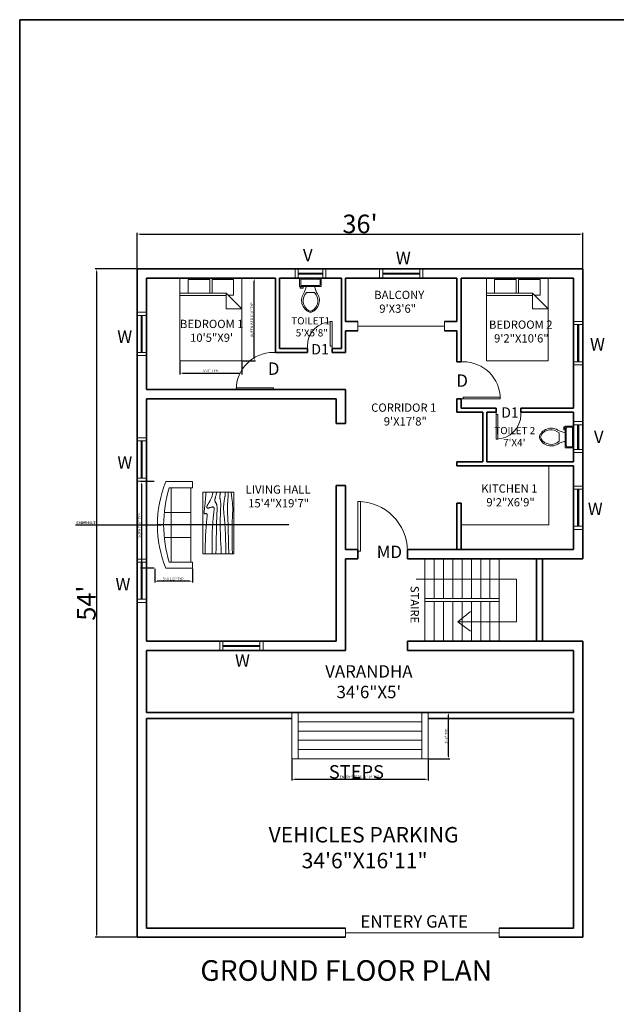
# Model space of a CAD drawing. Units: inches. Extents: x 2391 to 16591, y 7259 to 10239.
# Tile 19 of 27: x 2391 to 2970, y 9285 to 10239. Entities that reach past the tile are written whole.
import ezdxf

# ---------------------------------------------------------------- set-up
doc = ezdxf.new("R2010")
doc.units = ezdxf.units.IN
for name, color, linetype, lineweight in [('A-ANNO-DIMS', 4, 'Continuous', 18), ('A-ANNO-IDEN', 2, 'Continuous', 18), ('A-ANNO-SYMB', 3, 'Continuous', 18), ('A-ANNO-TITL', 3, 'Continuous', 30), ('A-ANNO-TTLB', 7, 'Continuous', 35), ('A-AREA-IDEN', 7, 'Continuous', 18), ('A-DOOR', 3, 'Continuous', 18), ('A-FLOR-CASE', 6, 'Continuous', 18), ('A-FLOR-FIXT', 9, 'Continuous', 18), ('A-FLOR-HRAL', 8, 'Continuous', 18), ('A-FLOR-STRS', 7, 'Continuous', 18), ('A-FURN', 8, 'Continuous', 18), ('A-GLAZ', 4, 'Continuous', 18), ('A-WALL', 7, 'Continuous', 35)]:
    doc.layers.add(name, color=color, linetype=linetype, lineweight=lineweight)
doc.styles.get("Standard").update_dxf_attribs({"font": 'arial.ttf'})
doc.dimstyles.new('ISO-25', dxfattribs={"dimtxt": 2.5, "dimasz": 2.5, "dimexe": 1.25, "dimexo": 0.625, "dimtad": 1, "dimdec": 0, "dimlunit": 3, "dimtxsty": 'Standard', "dimcen": 2.5, "dimadec": 0, "dimazin": 0, "dimtfac": 1, "dimtdec": 0, "dimtmove": 0, "dimatfit": 3, "dimfxl": 1, "dimarcsym": 0})

# ---------------------------------------------------------------- blocks, each defined once
blk = doc.blocks.new('*U11')
for p, q in [((-36, 0), (-36, 6)), ((0, 0), (0, 6))]:
    blk.add_line(p, q)
blk.add_lwpolyline([(0, 0), (0, -36), (-1.75, -36), (-1.75, 0)], close=True)
blk.add_arc((0, 0), 36, 180, 270)
blk = doc.blocks.new('*U8')
for p, q in [((-24, 0), (-24, -6)), ((0, 0), (0, -6))]:
    blk.add_line(p, q)
blk.add_lwpolyline([(0, 0), (0, 24), (-1.75, 24), (-1.75, 0)], close=True)
blk.add_arc((0, 0), 24, 90, 180)
blk = doc.blocks.new('*U12')
for p, q in [((0, 0), (0, -6)), ((-36, 0), (-36, -6))]:
    blk.add_line(p, q)
blk.add_lwpolyline([(0, 0), (0, 36), (-1.75, 36), (-1.75, 0)], close=True)
blk.add_arc((0, 0), 36, 90, 180)
blk = doc.blocks.new('*U9')
for p, q in [((0, 0), (0, 6)), ((24, 0), (24, 6))]:
    blk.add_line(p, q)
blk.add_lwpolyline([(0, 0), (0, -24), (1.75, -24), (1.75, 0)], close=True)
blk.add_arc((0, 0), 24, 270, 0)
blk = doc.blocks.new('*U18')
for p, q in [((0, 0), (0, -5)), ((32, 0), (32, -5))]:
    blk.add_line(p, q)
blk.add_lwpolyline([(0, 0), (0, 32), (1.75, 32), (1.75, 0)], close=True)
blk.add_arc((0, 0), 32, 0, 90)
blk = doc.blocks.new('Bed - Queen')
for p, q in [((0, -80.00003), (0, 0)), ((0, 0), (59.99999, 0)), ((59.99999, 0), (59.99999, -80.00003)), ((7.99999, -1.2), (28.79998, -1.2)), ((7.99999, -14.4), (7.99999, -1.2)), ((28.79998, -1.2), (28.79998, -14.4)), ((31.19999, -1.2), (51.99999, -1.2)), ((31.19999, -14.4), (31.19999, -1.2)), ((51.99999, -1.2), (51.99999, -16.4)), ((0, -14.4), (44.8, -14.4)), ((44.8, -16.8), (0, -16.8)), ((59.99999, -29.6), (44.8, -14.4)), ((44.8, -14.4), (44.8, -29.6)), ((51.99999, -16.4), (46.79936, -16.4)), ((44.8, -29.6), (59.99999, -29.6)), ((59.99999, -80.00003), (0, -80.00003))]:
    blk.add_line(p, q)
blk = doc.blocks.new('Toilet - top')
for p, q in [((-10, -8.5), (-8, -8.5)), ((-10, -9.5), (-10, -8.5)), ((-7, -9.5), (-10, -9.5)), ((-8, -8.5), (-8, -8)), ((-7, -8), (-7, -9.5)), ((-4, -8), (-6, -14)), ((4, -8), (6, -14)), ((9.5, -6), (9.5, -2)), ((4, -14), (-4, -14))]:
    blk.add_line(p, q)
blk.add_lwpolyline([(10.5, -8), (10.5, 0), (-10.5, 0), (-10.5, -8)], close=True)
for points in [[(-9.5, -2), (-9.5, -6)], [(8.5, -1), (-8.5, -1)], [(-8.5, -7), (8.5, -7)]]:
    blk.add_lwpolyline(points)
for centre, radius, start, end in [((-8.62, -1.88), 0.884, 81.8699, 188.1301), ((-8.62, -6.12), 0.884, 171.8699, 278.1301), ((8.62, -1.88), 0.884, 351.8699, 98.1301), ((8.62, -6.12), 0.884, 261.8699, 8.1301), ((3.52, -21.58), 12.17, 141.46911, 247.97143), ((4.2, -21.82), 11.33, 136.36773, 238.94682), ((-3.52, -21.58), 12.17, 292.02843, 38.53071), ((-4.2, -21.82), 11.33, 301.05301, 43.63209), ((0, -27.88), 4, 245.73182, 294.26817), ((0, -29), 4, 254.86053, 285.13947)]:
    blk.add_arc(centre, radius, start, end)
blk = doc.blocks.new('Sofa - Roundback 7 ft.')
for p, q in [((-12.00002, -32.4421), (-12.00003, -6.5971)), ((11.99997, -32.4421), (11.99998, -6.5971)), ((-36.000027, -34), (-36.000027, -11.4696)), ((-35.999844, -13.3819), (35.9998, -13.3819)), ((35.99998, -34), (35.99998, -11.4696)), ((-36.000027, -32.4421), (35.99998, -32.4421))]:
    blk.add_line(p, q)
for points in [[(-36.000027, -34), (-42.000027, -34), (-42.000027, -8)], [(41.99998, -8), (41.99998, -34), (35.99998, -34)]]:
    blk.add_lwpolyline(points)
for centre, radius, start, end in [((0, -114.25), 114.25, 68.43141, 111.5686), ((-0.00001, -127.1968), 121.1968, 72.72033, 107.2797)]:
    blk.add_arc(centre, radius, start, end)
blk = doc.blocks.new('Table - Rectangular Woodgrain 60 x 30 in.')
for p, q in [((0, 0), (0, -30)), ((60, 0), (0, 0)), ((60, -30), (60, 0)), ((0, -30), (60, -30))]:
    blk.add_line(p, q)
for points in [[(0, -2.4), (4.8155, -2.418), (9.0302, -2.4688), (12.709, -2.5477), (15.9167, -2.65), (18.7181, -2.7711), (21.1781, -2.9063), (23.3616, -3.0508), (25.3333, -3.2), (27.1477, -3.3495), (28.8172, -3.4958), (30.3437, -3.636), (31.7291, -3.7667), (32.9756, -3.8849), (34.0849, -3.9875), (35.059, -4.0714), (35.9, -4.1334), (36.6114, -4.1711), (37.2041, -4.1854), (37.6906, -4.1779), (38.0833, -4.15), (38.3948, -4.1034), (38.6375, -4.0396), (38.8239, -3.9602), (38.9666, -3.8667), (39.0764, -3.7608), (39.1573, -3.6448), (39.2116, -3.521), (39.2416, -3.3917), (39.2498, -3.2593), (39.2385, -3.1261), (39.21, -2.9944), (39.1666, -2.8667), (39.111, -2.7447), (39.0468, -2.6281), (38.978, -2.5163), (38.9083, -2.4083), (38.8418, -2.3035), (38.7823, -2.201), (38.7337, -2.1001), (38.7, -2), (38.6844, -1.9003), (38.6875, -1.8021), (38.7094, -1.707), (38.75, -1.6167), (38.8094, -1.5326), (38.8875, -1.4563), (38.9844, -1.3893), (39.1, -1.3333), (39.2351, -1.2896), (39.3937, -1.2583), (39.5804, -1.2396), (39.8, -1.2333), (40.057, -1.2396), (40.3562, -1.2583), (40.7023, -1.2896), (41.1, -1.3333), (41.5547, -1.3895), (42.0755, -1.4573), (42.6721, -1.5361), (43.3542, -1.625), (44.1316, -1.7233), (45.014, -1.8302), (46.0114, -1.9449), (47.1333, -2.0667), (48.3862, -2.1947), (49.7625, -2.3281), (51.2513, -2.4663), (52.8416, -2.6083), (54.5226, -2.7535), (56.2833, -2.9011), (58.1127, -3.0501), (60, -3.2)], [(0, -9.2), (6.5759, -9.0858), (11.9385, -9.0365), (16.2527, -9.0418), (19.6833, -9.0917), (22.3952, -9.1759), (24.5531, -9.2844), (26.322, -9.4069), (27.8666, -9.5333), (29.3241, -9.6553), (30.7203, -9.7719), (32.0532, -9.8837), (33.3208, -9.9917), (34.5213, -10.0965), (35.6526, -10.199), (36.7128, -10.2999), (37.7, -10.4), (38.6129, -10.4996), (39.4531, -10.5969), (40.223, -10.6895), (40.925, -10.775), (41.5613, -10.8512), (42.1344, -10.9156), (42.6465, -10.966), (43.1, -11), (43.4976, -11.0158), (43.8437, -11.0136), (44.143, -10.9942), (44.4, -10.9583), (44.6195, -10.9069), (44.8062, -10.8406), (44.9648, -10.7603), (45.1, -10.6667), (45.2155, -10.5598), (45.3114, -10.4365), (45.3871, -10.2929), (45.4416, -10.125), (45.4743, -9.929), (45.4844, -9.7011), (45.4709, -9.4371), (45.4333, -9.1333), (45.3716, -8.7883), (45.2896, -8.4104), (45.1919, -8.0107), (45.0833, -7.6), (44.9685, -7.1893), (44.8521, -6.7896), (44.7388, -6.4117), (44.6333, -6.0667), (44.54, -5.7628), (44.4614, -5.4979), (44.4001, -5.2675), (44.3583, -5.0667), (44.3384, -4.8909), (44.3427, -4.7354), (44.3736, -4.5956), (44.4333, -4.4667), (44.5236, -4.3453), (44.6427, -4.2333), (44.7884, -4.1339), (44.9583, -4.05), (45.1501, -3.9849), (45.3614, -3.9417), (45.59, -3.9234), (45.8333, -3.9333), (46.0915, -3.9749), (46.3734, -4.0531), (46.6906, -4.1736), (47.0542, -4.3417), (47.4756, -4.5629), (47.9661, -4.8427), (48.5372, -5.1866), (49.2, -5.6), (49.9676, -6.0844), (50.8594, -6.625), (51.8965, -7.2031), (53.1, -7.8), (54.491, -8.3969), (56.0906, -8.975), (57.9199, -9.5156), (60, -10)], [(0, -12.8), (5.1847, -12.9322), (9.6213, -13.0323), (13.3963, -13.1059), (16.5958, -13.1583), (19.3063, -13.1952), (21.614, -13.2219), (23.6054, -13.2439), (25.3666, -13.2667), (26.9728, -13.2947), (28.4531, -13.3281), (29.8256, -13.3663), (31.1083, -13.4083), (32.3191, -13.4535), (33.476, -13.501), (34.597, -13.5501), (35.7, -13.6), (36.7984, -13.6497), (37.8875, -13.6979), (38.9578, -13.743), (40, -13.7833), (41.0047, -13.8174), (41.9625, -13.8438), (42.864, -13.8607), (43.7, -13.8667), (44.4631, -13.8604), (45.1552, -13.8417), (45.7801, -13.8104), (46.3416, -13.7667), (46.8439, -13.7104), (47.2906, -13.6417), (47.6858, -13.5604), (48.0333, -13.4667), (48.3375, -13.3608), (48.6042, -13.2448), (48.8396, -13.121), (49.05, -12.9917), (49.2417, -12.8593), (49.4208, -12.7261), (49.5937, -12.5944), (49.7667, -12.4667), (49.9452, -12.3451), (50.1323, -12.2313), (50.3303, -12.1268), (50.5416, -12.0333), (50.7686, -11.9524), (51.0135, -11.8854), (51.2788, -11.8341), (51.5666, -11.8), (51.8785, -11.7843), (52.2116, -11.7865), (52.562, -11.8059), (52.926, -11.8417), (53.2998, -11.8931), (53.6795, -11.9594), (54.0614, -12.0397), (54.4416, -12.1333), (54.8223, -12.2401), (55.2293, -12.3625), (55.6942, -12.5037), (56.2489, -12.6667), (56.9251, -12.8547), (57.7545, -13.0708), (58.7689, -13.3182), (60, -13.6)], [(0, -18), (5.124, -17.7273), (9.6609, -17.5057), (13.6705, -17.3303), (17.2125, -17.1958), (20.3467, -17.0973), (23.1328, -17.0297), (25.6307, -16.9878), (27.9, -16.9667), (29.9928, -16.9617), (31.9302, -16.9703), (33.7254, -16.9907), (35.3917, -17.0208), (36.9423, -17.0588), (38.3906, -17.1026), (39.7499, -17.1503), (41.0333, -17.2), (42.2519, -17.2496), (43.4073, -17.2969), (44.4986, -17.3395), (45.525, -17.375), (46.4858, -17.4012), (47.3802, -17.4156), (48.2074, -17.416), (48.9667, -17.4), (49.6583, -17.3662), (50.2872, -17.3167), (50.8595, -17.2547), (51.3812, -17.1833), (51.8584, -17.1057), (52.2971, -17.025), (52.7034, -16.9443), (53.0833, -16.8667), (53.443, -16.7951), (53.789, -16.7313), (54.128, -16.6768), (54.4666, -16.6334), (54.8115, -16.6024), (55.1693, -16.5854), (55.5465, -16.5841), (55.95, -16.6), (56.3828, -16.6337), (56.8346, -16.6823), (57.2915, -16.7418), (57.7396, -16.8084), (58.165, -16.878), (58.5539, -16.9469), (58.8924, -17.0111), (59.1666, -17.0667), (59.3679, -17.1107), (59.5078, -17.1438), (59.6032, -17.1675), (59.6708, -17.1833), (59.7275, -17.193), (59.7901, -17.1979), (59.8753, -17.1998), (60, -17.2)], [(0, -22.4), (8.0098, -22.2501), (14.4094, -22.1011), (19.4168, -21.9535), (23.25, -21.8083), (26.1269, -21.6663), (28.2656, -21.5281), (29.884, -21.3947), (31.2, -21.2667), (32.3967, -21.1448), (33.5172, -21.0292), (34.5697, -20.9198), (35.5625, -20.8167), (36.5037, -20.7198), (37.4015, -20.6292), (38.2642, -20.5448), (39.1, -20.4667), (39.9164, -20.3951), (40.7187, -20.3313), (41.5117, -20.2768), (42.3, -20.2333), (43.0883, -20.2024), (43.8812, -20.1854), (44.6836, -20.1841), (45.5, -20.2), (46.3328, -20.234), (47.1747, -20.2844), (48.0163, -20.3488), (48.8479, -20.425), (49.66, -20.5106), (50.4429, -20.6031), (51.1872, -20.7004), (51.8833, -20.8), (52.5246, -20.8999), (53.1166, -20.9995), (53.6681, -21.0983), (54.1875, -21.1958), (54.6834, -21.2919), (55.1646, -21.3859), (55.6394, -21.4777), (56.1167, -21.5667), (56.6028, -21.6515), (57.0961, -21.7266), (57.5929, -21.7852), (58.0896, -21.8208), (58.5823, -21.8268), (59.0674, -21.7964), (59.5412, -21.723), (60, -21.6)], [(0, -25.2), (8.6355, -25.0504), (15.7026, -24.9031), (21.4049, -24.7606), (25.9458, -24.625), (29.529, -24.4988), (32.3578, -24.3844), (34.6359, -24.284), (36.5667, -24.2), (38.3213, -24.1341), (39.9417, -24.0854), (41.437, -24.0523), (42.8167, -24.0333), (44.0901, -24.0268), (45.2667, -24.0313), (46.3557, -24.0451), (47.3667, -24.0667), (48.309, -24.0947), (49.1928, -24.1287), (50.0284, -24.168), (50.826, -24.2125), (51.5959, -24.2617), (52.3483, -24.3151), (53.0935, -24.3725), (53.8417, -24.4334), (54.6009, -24.497), (55.3699, -24.561), (56.1454, -24.6226), (56.9239, -24.6792), (57.7021, -24.7279), (58.4764, -24.7662), (59.2435, -24.7911), (60, -24.8)], [(0, -28.8), (5.6867, -28.6681), (10.45, -28.5698), (14.407, -28.5012), (17.675, -28.4584), (20.3711, -28.4374), (22.6125, -28.4344), (24.5164, -28.4455), (26.2, -28.4667), (27.762, -28.4947), (29.2276, -28.5281), (30.6033, -28.5663), (31.8958, -28.6084), (33.1118, -28.6535), (34.2578, -28.7011), (35.3405, -28.7501), (36.3666, -28.8), (37.3443, -28.8497), (38.288, -28.8974), (39.2137, -28.9412), (40.1375, -28.9792), (41.0753, -29.0093), (42.0432, -29.0297), (43.0572, -29.0384), (44.1333, -29.0333), (45.2936, -29.0114), (46.5843, -28.9641), (48.0579, -28.8816), (49.7666, -28.7542), (51.7629, -28.5721), (54.0989, -28.3255), (56.8272, -28.0048), (60, -27.6)]]:
    blk.add_lwpolyline(points)
blk = doc.blocks.new('*D19')
at = {"layer": 'A-ANNO-DIMS', "color": 0, "lineweight": -2, "transparency": 16777216}
for p, q in [((2505.16, 9998.38), (2505.16, 10032.8)), ((2937.16, 9998.38), (2937.16, 10032.8)), ((2507.66, 10031.55), (2934.66, 10031.55))]:
    blk.add_line(p, q, dxfattribs=at)
at = {"layer": 'A-ANNO-DIMS', "color": 0, "transparency": 16777216}
for points in [[(2507.66, 10031.97), (2507.66, 10031.14), (2505.16, 10031.55)], [(2934.66, 10031.97), (2934.66, 10031.14), (2937.16, 10031.55)]]:
    blk.add_solid(points, dxfattribs=at)
at = {"layer": 'Defpoints', "color": 0, "transparency": 16777216}
for p in [(2937.16, 10031.55), (2505.16, 9997.76), (2937.16, 9997.76)]:
    blk.add_point(p, dxfattribs=at)
at = {"layer": 'A-ANNO-DIMS', "color": 0, "transparency": 16777216, "insert": (2721.16, 10041.38), "char_height": 2.5, "attachment_point": 5}
blk.add_mtext("{\\H7.2x;36'}", dxfattribs=at)
blk = doc.blocks.new('*D20')
at = {"layer": 'A-ANNO-DIMS', "color": 0, "lineweight": -2, "transparency": 16777216}
for p, q in [((2504.54, 9997.76), (2464.45, 9997.76)), ((2465.7, 9995.26), (2465.7, 9352.26)), ((2504.54, 9349.76), (2464.45, 9349.76))]:
    blk.add_line(p, q, dxfattribs=at)
at = {"layer": 'A-ANNO-DIMS', "color": 0, "transparency": 16777216}
for points in [[(2465.28, 9995.26), (2466.11, 9995.26), (2465.7, 9997.76)], [(2465.28, 9352.26), (2466.11, 9352.26), (2465.7, 9349.76)]]:
    blk.add_solid(points, dxfattribs=at)
at = {"layer": 'Defpoints', "color": 0, "transparency": 16777216}
for p in [(2505.16, 9997.76), (2465.7, 9349.76), (2505.16, 9349.76)]:
    blk.add_point(p, dxfattribs=at)
at = {"layer": 'A-ANNO-DIMS', "color": 0, "transparency": 16777216, "insert": (2455.92, 9673.76), "char_height": 2.5, "attachment_point": 5, "rotation": 90}
blk.add_mtext("{\\H7.2x;54'}", dxfattribs=at)
blk = doc.blocks.new('WINDOW-36-PLAN')
for p, q in [((9, 42), (0, 42)), ((9, 39), (0, 39)), ((4, 39), (4, 3)), ((4.5, 39), (4.5, 3)), ((5, 39), (5, 3)), ((9, 3), (0, 3)), ((9, 0), (0, 0))]:
    blk.add_line(p, q)
blk = doc.blocks.new('VENT-24-PLAN')
for p, q in [((9, 30), (0, 30)), ((9, 27), (0, 27)), ((4, 27), (4, 3)), ((4.5, 27), (4.5, 3)), ((5, 27), (5, 3)), ((9, 3), (0, 3)), ((9, 0), (0, 0))]:
    blk.add_line(p, q)
blk = doc.blocks.new('STAIR-RETURN-FLIGHT')
for p, q in [((0, 80), (0, 0)), ((9, 80), (9, 41.5)), ((18, 80), (18, 41.5)), ((27, 80), (27, 41.5)), ((36, 80), (36, 41.5)), ((45, 80), (45, 41.5)), ((54, 80), (54, 41.5)), ((63, 80), (63, 41.5)), ((72, 80), (72, 0)), ((72, 41.5), (0, 41.5)), ((72, 38.5), (0, 38.5)), ((9, 38.5), (9, 0)), ((18, 38.5), (18, 0)), ((27, 38.5), (27, 0)), ((36, 38.5), (36, 0)), ((45, 38.5), (45, 0)), ((54, 38.5), (54, 0)), ((63, 38.5), (63, 0))]:
    blk.add_line(p, q)
blk = doc.blocks.new('STAIR-DIRECTION-ARROW')
for p, q in [((0, 50.31), (97.37, 50.31)), ((97.37, 50.31), (97.37, 8.81)), ((40.34, 8.81), (52.74, 18.89)), ((97.37, 8.81), (40.34, 8.81)), ((40.34, 8.81), (52.74, 0))]:
    blk.add_line(p, q)
blk = doc.blocks.new('COUNTER-L-KITCHEN-TYPE2')
for p in [(85, 57), (0, 0)]:
    blk.add_line(p, (85, 0))
blk = doc.blocks.new('STAIR-ENTRY-STEPS')
for p, q in [((0, 45), (0, 0)), ((6, 45), (6, 0)), ((126, 45), (126, 0)), ((132, 45), (132, 0)), ((6, 36), (126, 36)), ((6, 27), (126, 27)), ((6, 18), (126, 18)), ((6, 9), (126, 9)), ((0, 0), (132, 0))]:
    blk.add_line(p, q)
blk = doc.blocks.new('*D45')
at = {"layer": 'A-ANNO-DIMS', "color": 0, "lineweight": -2, "transparency": 16777216}
for p, q in [((2607.29, 9988.76), (2619.91, 9988.76)), ((2618.66, 9911.26), (2618.66, 9986.26)), ((2607.29, 9908.76), (2619.91, 9908.76))]:
    blk.add_line(p, q, dxfattribs=at)
at = {"layer": 'A-ANNO-DIMS', "color": 0, "transparency": 16777216}
for points in [[(2618.24, 9986.26), (2619.08, 9986.26), (2618.66, 9988.76)], [(2618.24, 9911.26), (2619.08, 9911.26), (2618.66, 9908.76)]]:
    blk.add_solid(points, dxfattribs=at)
at = {"layer": 'Defpoints', "color": 0, "transparency": 16777216}
for p in [(2606.66, 9988.76), (2618.66, 9988.76), (2606.66, 9908.76)]:
    blk.add_point(p, dxfattribs=at)
at = {"layer": 'A-ANNO-DIMS', "color": 0, "transparency": 16777216, "insert": (2616.67, 9948.76), "char_height": 2.5, "attachment_point": 5, "rotation": 90}
blk.add_mtext('QUEEN BED 6\'-8" TYP.', dxfattribs=at)
blk = doc.blocks.new('*D46')
at = {"layer": 'A-ANNO-DIMS', "color": 0, "lineweight": -2, "transparency": 16777216}
for p, q in [((2546.66, 9908.13), (2546.66, 9895.51)), ((2606.66, 9908.13), (2606.66, 9895.51)), ((2549.16, 9896.76), (2604.16, 9896.76))]:
    blk.add_line(p, q, dxfattribs=at)
at = {"layer": 'A-ANNO-DIMS', "color": 0, "transparency": 16777216}
for points in [[(2549.16, 9897.17), (2549.16, 9896.34), (2546.66, 9896.76)], [(2604.16, 9897.17), (2604.16, 9896.34), (2606.66, 9896.76)]]:
    blk.add_solid(points, dxfattribs=at)
at = {"layer": 'Defpoints', "color": 0, "transparency": 16777216}
for p in [(2546.66, 9908.76), (2606.66, 9908.76), (2606.66, 9896.76)]:
    blk.add_point(p, dxfattribs=at)
at = {"layer": 'A-ANNO-DIMS', "color": 0, "transparency": 16777216, "insert": (2576.66, 9898.66), "char_height": 2.5, "attachment_point": 5}
blk.add_mtext('5\'-0" TYP.', dxfattribs=at)
blk = doc.blocks.new('*D49')
at = {"layer": 'A-ANNO-DIMS', "color": 0, "lineweight": -2, "transparency": 16777216}
for p, q in [((2521.54, 9791.53), (2508.32, 9791.53)), ((2509.57, 9710.03), (2509.57, 9789.03)), ((2521.54, 9707.53), (2508.32, 9707.53))]:
    blk.add_line(p, q, dxfattribs=at)
at = {"layer": 'A-ANNO-DIMS', "color": 0, "transparency": 16777216}
for points in [[(2509.15, 9789.03), (2509.98, 9789.03), (2509.57, 9791.53)], [(2509.15, 9710.03), (2509.98, 9710.03), (2509.57, 9707.53)]]:
    blk.add_solid(points, dxfattribs=at)
at = {"layer": 'Defpoints', "color": 0, "transparency": 16777216}
for p in [(2509.57, 9791.53), (2522.17, 9791.53), (2522.17, 9707.53)]:
    blk.add_point(p, dxfattribs=at)
at = {"layer": 'A-ANNO-DIMS', "color": 0, "transparency": 16777216, "insert": (2507.65, 9749.53), "char_height": 2.5, "attachment_point": 5, "rotation": 90}
blk.add_mtext('SOFA 7\'-0" TYP.', dxfattribs=at)
blk = doc.blocks.new('*D50')
at = {"layer": 'A-ANNO-DIMS', "color": 0, "lineweight": -2, "transparency": 16777216}
for p, q in [((2522.17, 9706.91), (2522.17, 9693.68)), ((2558.83, 9706.91), (2558.83, 9693.68)), ((2556.33, 9694.93), (2524.67, 9694.93))]:
    blk.add_line(p, q, dxfattribs=at)
at = {"layer": 'A-ANNO-DIMS', "color": 0, "transparency": 16777216}
for points in [[(2524.67, 9695.35), (2524.67, 9694.52), (2522.17, 9694.93)], [(2556.33, 9695.35), (2556.33, 9694.52), (2558.83, 9694.93)]]:
    blk.add_solid(points, dxfattribs=at)
at = {"layer": 'Defpoints', "color": 0, "transparency": 16777216}
for p in [(2522.17, 9707.53), (2558.83, 9707.53), (2522.17, 9694.93)]:
    blk.add_point(p, dxfattribs=at)
at = {"layer": 'A-ANNO-DIMS', "color": 0, "transparency": 16777216, "insert": (2540.5, 9696.85), "char_height": 2.5, "attachment_point": 5}
blk.add_mtext('3\'-0 1/2" TYP.', dxfattribs=at)
blk = doc.blocks.new('*D61')
at = {"layer": 'A-ANNO-DIMS', "color": 0, "lineweight": -2, "transparency": 16777216}
for p, q in [((2655.16, 9522.13), (2655.16, 9501.71)), ((2787.16, 9522.13), (2787.16, 9501.71)), ((2657.66, 9502.96), (2784.66, 9502.96))]:
    blk.add_line(p, q, dxfattribs=at)
at = {"layer": 'A-ANNO-DIMS', "color": 0, "transparency": 16777216}
for points in [[(2657.66, 9503.37), (2657.66, 9502.54), (2655.16, 9502.96)], [(2784.66, 9503.37), (2784.66, 9502.54), (2787.16, 9502.96)]]:
    blk.add_solid(points, dxfattribs=at)
at = {"layer": 'Defpoints', "color": 0, "transparency": 16777216}
for p in [(2655.16, 9522.76), (2787.16, 9522.76), (2787.16, 9502.96)]:
    blk.add_point(p, dxfattribs=at)
at = {"layer": 'A-ANNO-DIMS', "color": 0, "transparency": 16777216, "insert": (2721.16, 9504.88), "char_height": 2.5, "attachment_point": 5}
blk.add_mtext('ENTRY STEPS 11\'-0" TYP.', dxfattribs=at)
blk = doc.blocks.new('*D62')
at = {"layer": 'A-ANNO-DIMS', "color": 0, "lineweight": -2, "transparency": 16777216}
for p, q in [((2787.79, 9567.76), (2808.21, 9567.76)), ((2806.96, 9525.26), (2806.96, 9565.26)), ((2787.79, 9522.76), (2808.21, 9522.76))]:
    blk.add_line(p, q, dxfattribs=at)
at = {"layer": 'A-ANNO-DIMS', "color": 0, "transparency": 16777216}
for points in [[(2806.54, 9565.26), (2807.38, 9565.26), (2806.96, 9567.76)], [(2806.54, 9525.26), (2807.38, 9525.26), (2806.96, 9522.76)]]:
    blk.add_solid(points, dxfattribs=at)
at = {"layer": 'Defpoints', "color": 0, "transparency": 16777216}
for p in [(2787.16, 9567.76), (2806.96, 9567.76), (2787.16, 9522.76)]:
    blk.add_point(p, dxfattribs=at)
at = {"layer": 'A-ANNO-DIMS', "color": 0, "transparency": 16777216, "insert": (2805.06, 9545.26), "char_height": 2.5, "attachment_point": 5, "rotation": 90}
blk.add_mtext('3\'-9" TYP.', dxfattribs=at)
blk = doc.blocks.new('*D117')
at = {"layer": 'A-ANNO-DIMS', "color": 0, "lineweight": -2, "transparency": 16777216}
for p, q in [((2449.31, 9749.53), (2528.33, 9749.53)), ((2652.03, 9749.53), (2530.83, 9749.53))]:
    blk.add_line(p, q, dxfattribs=at)
at = {"layer": 'A-ANNO-DIMS', "color": 0, "transparency": 16777216}
blk.add_solid([(2528.33, 9749.95), (2528.33, 9749.11), (2530.83, 9749.53)], dxfattribs=at)
at = {"layer": 'Defpoints', "color": 0, "transparency": 16777216}
for p in [(2530.83, 9749.53), (2652.03, 9749.53)]:
    blk.add_point(p, dxfattribs=at)
at = {"layer": 'A-ANNO-DIMS', "color": 0, "transparency": 16777216, "insert": (2458.11, 9751.43), "char_height": 2.5, "attachment_point": 5, "rotation": 0.00135}
blk.add_mtext('6X R10\'-1"', dxfattribs=at)
blk = doc.blocks.new('*D118')
at = {"layer": 'A-ANNO-DIMS', "color": 0, "lineweight": -2, "transparency": 16777216}
for p, q in [((2445.53, 9749.53), (2522.33, 9749.53)), ((2639.08, 9749.53), (2524.83, 9749.53))]:
    blk.add_line(p, q, dxfattribs=at)
at = {"layer": 'A-ANNO-DIMS', "color": 0, "transparency": 16777216}
blk.add_solid([(2522.33, 9749.95), (2522.33, 9749.11), (2524.83, 9749.53)], dxfattribs=at)
at = {"layer": 'Defpoints', "color": 0, "transparency": 16777216}
for p in [(2524.83, 9749.53), (2639.08, 9749.53)]:
    blk.add_point(p, dxfattribs=at)
at = {"layer": 'A-ANNO-DIMS', "color": 0, "transparency": 16777216, "insert": (2456.28, 9751.45), "char_height": 2.5, "attachment_point": 5, "rotation": 0.00144}
blk.add_mtext('6X R9\'-6 1/2"', dxfattribs=at)

msp = doc.modelspace()

# ---------------------------------------------------------------- linework, layer by layer
at = {"layer": 'A-ANNO-TTLB'}
msp.add_lwpolyline([(2391.28, 10239.38), (4154.2, 10239.38), (4154.2, 7258.54), (2391.28, 7258.54)], close=True, dxfattribs=at)
at = {"layer": 'A-DOOR'}
for p, q in [((2707.16, 9358.76), (2707.16, 9349.76)), ((2856.16, 9358.76), (2856.16, 9349.76)), ((2707.16, 9354.26), (2856.16, 9354.26))]:
    msp.add_line(p, q, dxfattribs=at)
at = {"layer": 'A-FLOR-HRAL'}
for p, q in [((2719.16, 9937.76), (2719.16, 9946.76)), ((2803.16, 9937.76), (2803.16, 9946.76)), ((2719.16, 9942.26), (2803.16, 9942.26))]:
    msp.add_line(p, q, dxfattribs=at)
at = {"layer": 'A-WALL'}
for p, q in [((2505.16, 9997.76), (2937.16, 9997.76)), ((2505.16, 9349.76), (2505.16, 9997.76)), ((2937.16, 9997.76), (2937.16, 9716.76)), ((2514.16, 9988.76), (2639.16, 9988.76)), ((2514.16, 9880.76), (2514.16, 9988.76)), ((2639.16, 9916.76), (2639.16, 9988.76)), ((2643.16, 9920.76), (2643.16, 9988.76)), ((2643.16, 9988.76), (2703.16, 9988.76)), ((2703.16, 9920.76), (2703.16, 9988.76)), ((2707.16, 9988.76), (2815.16, 9988.76)), ((2707.16, 9946.76), (2707.16, 9988.76)), ((2815.16, 9946.76), (2815.16, 9988.76)), ((2819.16, 9988.76), (2928.16, 9988.76)), ((2819.16, 9907.76), (2819.16, 9988.76)), ((2928.16, 9988.76), (2928.16, 9862.76)), ((2707.16, 9946.76), (2719.16, 9946.76)), ((2803.16, 9946.76), (2815.16, 9946.76)), ((2707.16, 9916.76), (2707.16, 9937.76)), ((2707.16, 9937.76), (2719.16, 9937.76)), ((2803.16, 9937.76), (2815.16, 9937.76)), ((2815.16, 9907.76), (2815.16, 9937.76)), ((2643.16, 9920.76), (2670.16, 9920.76)), ((2670.16, 9916.76), (2670.16, 9920.76)), ((2694.16, 9916.76), (2694.16, 9920.76)), ((2694.16, 9920.76), (2703.16, 9920.76)), ((2639.16, 9916.76), (2670.16, 9916.76)), ((2694.16, 9916.76), (2707.16, 9916.76)), ((2815.16, 9907.76), (2819.16, 9907.76)), ((2514.16, 9880.76), (2707.16, 9880.76)), ((2707.16, 9847.76), (2707.16, 9880.76)), ((2514.16, 9871.76), (2698.16, 9871.76)), ((2514.16, 9636.76), (2514.16, 9871.76)), ((2698.16, 9847.76), (2698.16, 9871.76)), ((2815.16, 9858.76), (2815.16, 9871.76)), ((2815.16, 9871.76), (2819.16, 9871.76)), ((2819.16, 9862.76), (2819.16, 9871.76)), ((2819.16, 9862.76), (2853.16, 9862.76)), ((2853.16, 9862.76), (2853.16, 9858.76)), ((2877.16, 9862.76), (2877.16, 9858.76)), ((2877.16, 9862.76), (2928.16, 9862.76)), ((2815.16, 9858.76), (2840.16, 9858.76)), ((2840.16, 9858.76), (2840.16, 9810.76)), ((2844.16, 9858.76), (2844.16, 9810.76)), ((2844.16, 9858.76), (2853.16, 9858.76)), ((2877.16, 9858.76), (2928.16, 9858.76)), ((2928.16, 9858.76), (2928.16, 9810.76)), ((2698.16, 9847.76), (2707.16, 9847.76)), ((2815.16, 9810.76), (2840.16, 9810.76)), ((2815.16, 9806.76), (2815.16, 9810.76)), ((2815.16, 9806.76), (2928.16, 9806.76)), ((2844.16, 9810.76), (2928.16, 9810.76)), ((2928.16, 9806.76), (2928.16, 9725.76)), ((2698.16, 9636.76), (2698.16, 9787.76)), ((2698.16, 9787.76), (2707.16, 9787.76)), ((2707.16, 9725.76), (2707.16, 9787.76)), ((2815.16, 9725.76), (2815.16, 9770.76)), ((2815.16, 9770.76), (2819.16, 9770.76)), ((2819.16, 9725.76), (2819.16, 9770.76)), ((2707.16, 9725.76), (2719.16, 9725.76)), ((2719.16, 9716.76), (2719.16, 9725.76)), ((2767.16, 9716.76), (2767.16, 9725.76)), ((2767.16, 9725.76), (2928.16, 9725.76)), ((2707.16, 9627.76), (2707.16, 9716.76)), ((2707.16, 9716.76), (2719.16, 9716.76)), ((2767.16, 9716.76), (2937.16, 9716.76)), ((2892.16, 9716.76), (2892.16, 9636.76)), ((2898.16, 9716.76), (2898.16, 9636.76)), ((2514.16, 9636.76), (2698.16, 9636.76)), ((2767.16, 9636.76), (2937.16, 9636.76)), ((2767.16, 9627.76), (2767.16, 9636.76)), ((2937.16, 9636.76), (2937.16, 9349.76)), ((2514.16, 9627.76), (2707.16, 9627.76)), ((2514.16, 9567.76), (2514.16, 9627.76)), ((2767.16, 9627.76), (2928.16, 9627.76)), ((2928.16, 9627.76), (2928.16, 9567.76)), ((2514.16, 9567.76), (2707.16, 9567.76)), ((2514.16, 9567.76), (2928.16, 9567.76)), ((2514.16, 9358.76), (2514.16, 9561.76)), ((2514.16, 9561.76), (2655.16, 9561.76)), ((2787.16, 9561.76), (2928.16, 9561.76)), ((2928.16, 9561.76), (2928.16, 9358.76)), ((2707.16, 9358.76), (2514.16, 9358.76)), ((2928.16, 9358.76), (2856.16, 9358.76)), ((2707.16, 9349.76), (2505.16, 9349.76)), ((2937.16, 9349.76), (2856.16, 9349.76))]:
    msp.add_line(p, q, dxfattribs=at)

# ---------------------------------------------------------------- block references
at = {"layer": 'A-ANNO-SYMB'}
msp.add_blockref('STAIR-DIRECTION-ARROW', (2775.59, 9646.72), dxfattribs=at)
at = {"layer": 'A-DOOR'}
for name, p in [('*U8', (2694.16, 9922.76)), ('*U9', (2853.16, 9856.76))]:
    msp.add_blockref(name, p, dxfattribs=at)
at = {"layer": 'A-DOOR', "rotation": 270}
for name, p in [('*U11', (2637.16, 9880.76)), ('*U12', (2821.16, 9871.76))]:
    msp.add_blockref(name, p, dxfattribs=at)
at = {"layer": 'A-DOOR', "xscale": 1.5, "yscale": 1.5, "zscale": 1.5}
msp.add_blockref('*U18', (2719.16, 9724.26), dxfattribs=at)
at = {"layer": 'A-FLOR-CASE'}
msp.add_blockref('COUNTER-L-KITCHEN-TYPE2', (2819.16, 9749.76), dxfattribs=at)
at = {"layer": 'A-FLOR-FIXT'}
msp.add_blockref('Toilet - top', (2673.16, 9988.76), dxfattribs=at)
at = {"layer": 'A-FLOR-FIXT', "rotation": 270}
msp.add_blockref('Toilet - top', (2928.16, 9834.76), dxfattribs=at)
at = {"layer": 'A-FLOR-STRS', "rotation": 180}
msp.add_blockref('STAIR-RETURN-FLIGHT', (2856.16, 9716.76), dxfattribs=at)
at = {"layer": 'A-FLOR-STRS'}
msp.add_blockref('STAIR-ENTRY-STEPS', (2655.16, 9522.76), dxfattribs=at)
at = {"layer": 'A-FURN'}
for p in [(2546.66, 9988.76), (2843.66, 9988.76)]:
    msp.add_blockref('Bed - Queen', p, dxfattribs=at)
at = {"layer": 'A-FURN', "rotation": 90}
for name, p in [('Sofa - Roundback 7 ft.', (2524.83, 9749.53)), ('Table - Rectangular Woodgrain 60 x 30 in.', (2568.74, 9721.48))]:
    msp.add_blockref(name, p, dxfattribs=at)
at = {"layer": 'A-GLAZ'}
for name, p, rotation in [('VENT-24-PLAN', (2658.16, 9997.76), 270.0000000000127), ('WINDOW-36-PLAN', (2740.16, 9997.76), 270.0000000000149), ('WINDOW-36-PLAN', (2585.16, 9636.76), 269.9999999999958)]:
    msp.add_blockref(name, p, dxfattribs=dict(at, rotation=rotation))
for name, p in [('WINDOW-36-PLAN', (2505.16, 9913.76)), ('WINDOW-36-PLAN', (2928.16, 9904.76)), ('VENT-24-PLAN', (2928.16, 9819.76)), ('WINDOW-36-PLAN', (2505.16, 9792.01)), ('WINDOW-36-PLAN', (2928.16, 9745.26)), ('WINDOW-36-PLAN', (2505.16, 9674.51))]:
    msp.add_blockref(name, p, dxfattribs=at)

# ---------------------------------------------------------------- texts
at = {"layer": 'A-ANNO-IDEN', "attachment_point": 1}
for s, width, insert, char_height in [('V', 17.0712, (2665.85, 10017.08), 12), ('W', 41.0391, (2755.98, 10014.33), 12), ('W', 41.0391, (2485.92, 9938.07), 12), ('W', 41.0391, (2944.16, 9930.66), 12), ('D1', 88.0557, (2674.02, 9924.88), 10), ('D', 711.4851, (2631.84, 9907.07), 12), ('D', 711.4851, (2814.57, 9895.49), 12), ('D1', 88.0557, (2858.1, 9863.57), 10), ('V', 17.0712, (2947.91, 9840.96), 12), ('W', 41.0391, (2486.01, 9816.16), 12), ('W', 41.0391, (2942.03, 9771.11), 12), ('MD', 711.4851, (2737.4, 9729.45), 12), ('W', 41.0391, (2484.17, 9698.05), 12), ('W', 41.0391, (2600.07, 9624.01), 12)]:
    msp.add_mtext_dynamic_manual_height_columns(s, width=width, gutter_width=12.5, heights=[0], dxfattribs=dict(at, insert=insert, char_height=char_height))
at = {"layer": 'A-ANNO-TITL', "insert": (2566.38, 9327.59), "char_height": 20, "attachment_point": 1}
msp.add_mtext_dynamic_manual_height_columns('GROUND FLOOR PLAN', width=1223.5938, gutter_width=12.5, heights=[0], dxfattribs=at)
at = {"layer": 'A-AREA-IDEN', "attachment_point": 1}
for s, width, insert, char_height in [('BALCONY\\P  9\'X3\'6"', 125.309, (2734.97, 9976.58), 8), ('BEDROOM 1\\P    10\'5"X9\'', 152.4027, (2546.66, 9948.43), 8), ('TOILET1\\P  5\'X5\'8"', 175.2431, (2654.59, 9950.98), 7), ('BEDROOM 2\\P  9\'2"X10\'6"', 186.7643, (2846.22, 9947.75), 8), ('CORRIDOR 1\\P     9\'X17\'8"', 386.0733, (2732.01, 9867.29), 8), ("{\\H0.875x;TOILET 2\\P    7'X4}'", 130.8261, (2851.44, 9844.55), 8), ('LIVING HALL\\P 15\'4"X19\'7"', 316.1653, (2610.33, 9787.9), 8), ('KITCHEN 1\\P  9\'2"X6\'9"', 260.4884, (2838.76, 9788.87), 8), ('VARANDHA\\P   34\'6"X5\'', 463.6702, (2687.43, 9613.58), 12), ('{STEPS}', 155.1331, (2690.97, 9516.67), 13), ('VEHICLES PARKING\\P       34\'6"X16\'11"', 315.868, (2632.55, 9456.7), 15), ('ENTERY GATE', 133.1329, (2721.57, 9371.16), 12)]:
    msp.add_mtext_dynamic_manual_height_columns(s, width=width, gutter_width=12.5, heights=[0], dxfattribs=dict(at, insert=insert, char_height=char_height))
at = {"layer": 'A-AREA-IDEN', "insert": (2778.21, 9690.52), "char_height": 8, "attachment_point": 1, "rotation": 270}
msp.add_mtext_dynamic_manual_height_columns('STAIRE', width=212.5876, gutter_width=12.5, heights=[0], dxfattribs=at)

# ---------------------------------------------------------------- dimensions: what is measured, and where the dimension line sits
at = {"layer": 'A-ANNO-DIMS'}
for base, p1, p2, text, override, picture, middle in [((2937.16, 10031.55), (2505.16, 9997.76), (2937.16, 9997.76), '{\\H7.2x;<>}', {"dimclrd": 0, "dimclre": 0, "dimclrt": 0}, '*D19', (2721.16, 10041.38)), ((2606.66, 9896.76), (2546.66, 9908.76), (2606.66, 9908.76), '<> TYP.', {"dimdec": 1, "dimlfac": 1, "dimrnd": 0, "dimzin": 1, "dimdsep": 46, "dimlunit": 4, "dimfrac": 2}, '*D46', (2576.66, 9898.66)), ((2787.16, 9502.96), (2655.16, 9522.76), (2787.16, 9522.76), 'ENTRY STEPS <> TYP.', {"dimdec": 1, "dimlfac": 1, "dimrnd": 0, "dimzin": 1, "dimdsep": 46, "dimlunit": 4, "dimfrac": 2}, '*D61', (2721.16, 9504.88))]:
    dim = msp.add_linear_dim(base=base, p1=p1, p2=p2, text=text, dimstyle='ISO-25', override=override, dxfattribs=at)
    dim.commit()
    dim.dimension.update_dxf_attribs({"geometry": picture, "text_midpoint": middle})
for base, p1, p2, angle, text, override, picture, middle in [((2465.7, 9349.76), (2505.16, 9997.76), (2505.16, 9349.76), 90, '{\\H7.2x;<>}', {"dimclrd": 0, "dimclre": 0, "dimclrt": 0}, '*D20', (2455.92, 9673.76)), ((2618.66, 9988.76), (2606.66, 9908.76), (2606.66, 9988.76), 90, 'QUEEN BED <> TYP.', {"dimdec": 1, "dimlfac": 1, "dimrnd": 0, "dimzin": 1, "dimdsep": 46, "dimlunit": 4, "dimfrac": 2}, '*D45', (2616.67, 9948.76)), ((2509.57, 9791.53), (2522.17, 9707.53), (2522.17, 9791.53), 90, 'SOFA <> TYP.', {"dimdec": 1, "dimlfac": 1, "dimrnd": 0, "dimzin": 1, "dimdsep": 46, "dimlunit": 4, "dimfrac": 2}, '*D49', (2507.65, 9749.53)), ((2522.17, 9694.93), (2558.83, 9707.53), (2522.17, 9707.53), 180, '<> TYP.', {"dimdec": 1, "dimlfac": 1, "dimrnd": 0, "dimzin": 1, "dimdsep": 46, "dimlunit": 4, "dimfrac": 2}, '*D50', (2540.5, 9696.85)), ((2806.96, 9567.76), (2787.16, 9522.76), (2787.16, 9567.76), 90, '<> TYP.', {"dimdec": 1, "dimlfac": 1, "dimrnd": 0, "dimzin": 1, "dimdsep": 46, "dimlunit": 4, "dimfrac": 2}, '*D62', (2805.06, 9545.26))]:
    dim = msp.add_linear_dim(base=base, p1=p1, p2=p2, angle=angle, text=text, dimstyle='ISO-25', override=override, dxfattribs=at)
    dim.commit()
    dim.dimension.update_dxf_attribs({"geometry": picture, "text_midpoint": middle})
for center, mpoint, picture, middle in [((2639.08298, 9749.532873), (2524.83298, 9749.53), '*D118', (2456.28298002, 9749.5282762)), ((2652.03, 9749.53), (2530.83, 9749.53), '*D117', (2458.11, 9749.53))]:
    dim = msp.add_radius_dim(center=center, mpoint=mpoint, text='6X <>', dimstyle='ISO-25', override={"dimdec": 1, "dimlfac": 1, "dimrnd": 0, "dimzin": 1, "dimdsep": 46, "dimlunit": 4, "dimfrac": 2}, dxfattribs=at)
    dim.commit()
    dim.dimension.update_dxf_attribs({"geometry": picture, "text_midpoint": middle, "dimtype": 164})

doc.saveas('drawing.dxf')
